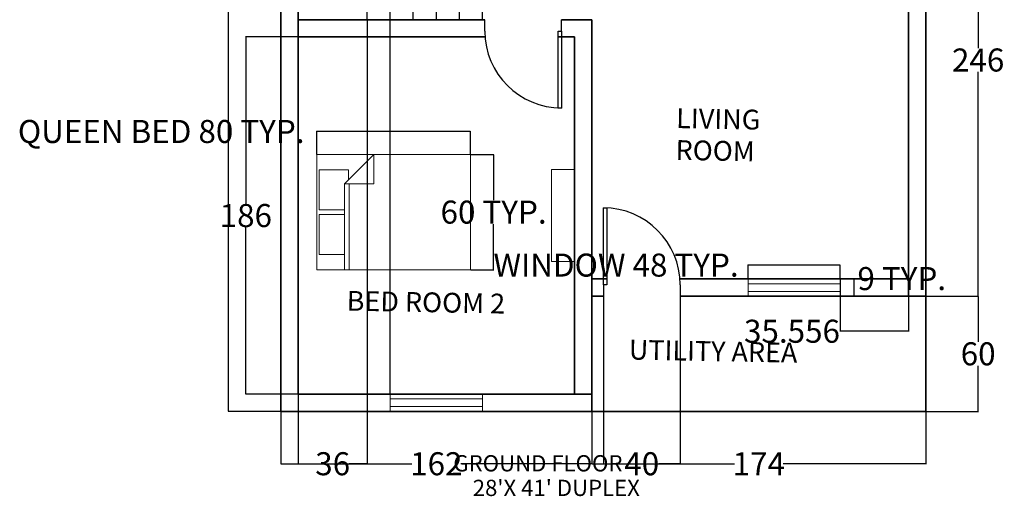
# Model space of a CAD drawing. Units: inches. Extents: x 424 to 1593, y 6 to 578.
# Tile 1 of 4: x 424 to 937, y 6 to 255. Entities that reach past the tile are written whole.
import ezdxf

# ---------------------------------------------------------------- set-up
doc = ezdxf.new("R2010")
doc.units = ezdxf.units.IN
doc.header["$MEASUREMENT"] = 0
for name, color, linetype, lineweight in [('A-ANNO-DIMS', 2, 'Continuous', 18), ('A-ANNO-TEXT', 7, 'Continuous', 25), ('A-AREA-IDEN', 7, 'Continuous', 18), ('A-DOOR', 3, 'Continuous', 25), ('A-FLOR-CASE', 9, 'Continuous', 18), ('A-FLOR-STRS', 7, 'Continuous', 25), ('A-FURN', 8, 'Continuous', 18), ('A-GLAZ', 4, 'Continuous', 18), ('A-WALL', 7, 'Continuous', 35)]:
    doc.layers.add(name, color=color, linetype=linetype, lineweight=lineweight)
doc.styles.get("Standard").update_dxf_attribs({"font": 'arial.ttf'})
doc.dimstyles.get("Standard").update_dxf_attribs({"dimtxt": 12, "dimasz": 0.18, "dimexe": 0.18, "dimexo": 0.0625, "dimgap": 0.09, "dimtad": 0, "dimtih": 1, "dimtoh": 1, "dimdec": 0, "dimzin": 0, "dimdsep": 46, "dimlunit": 3, "dimtxsty": 'Standard', "dimcen": 0.09, "dimadec": 0, "dimazin": 0, "dimtfac": 1, "dimtdec": 0, "dimtofl": 0, "dimtmove": 0, "dimatfit": 3, "dimfxl": 1, "dimtolj": 1, "dimtzin": 0, "dimarcsym": 0})

# ---------------------------------------------------------------- blocks, each defined once
blk = doc.blocks.new('*U4')
for p, q in [((-40, 0), (-40, 6)), ((0, 0), (0, 6))]:
    blk.add_line(p, q)
blk.add_lwpolyline([(0, 0), (0, -40), (-1.75, -40), (-1.75, 0)], close=True)
blk.add_arc((0, 0), 40, 180, 270)
blk = doc.blocks.new('*U6')
for p, q in [((0, 0), (0, -6)), ((40, 0), (40, -6))]:
    blk.add_line(p, q)
blk.add_lwpolyline([(0, 0), (0, 40), (1.75, 40), (1.75, 0)], close=True)
blk.add_arc((0, 0), 40, 0, 90)
blk = doc.blocks.new('Bed - Queen')
for p, q in [((0, -80.00003), (0, 0)), ((0, 0), (59.99999, 0)), ((59.99999, 0), (59.99999, -80.00003)), ((7.99999, -1.2), (28.79998, -1.2)), ((7.99999, -14.4), (7.99999, -1.2)), ((28.79998, -1.2), (28.79998, -14.4)), ((31.19999, -1.2), (51.99999, -1.2)), ((31.19999, -14.4), (31.19999, -1.2)), ((51.99999, -1.2), (51.99999, -16.4)), ((0, -14.4), (44.8, -14.4)), ((59.99999, -29.6), (44.8, -14.4)), ((44.8, -14.4), (44.8, -29.6)), ((44.8, -16.8), (0, -16.8)), ((51.99999, -16.4), (46.79936, -16.4)), ((44.8, -29.6), (59.99999, -29.6)), ((59.99999, -80.00003), (0, -80.00003))]:
    blk.add_line(p, q)
blk = doc.blocks.new('WIN-48IN')
for p, q in [((2.5, 48), (2.5, 0)), ((6.5, 48), (6.5, 0))]:
    blk.add_line(p, q)
blk.add_lwpolyline([(0, 48), (9, 48), (9, 0), (0, 0)], close=True)
blk = doc.blocks.new('STAIR-RETURN-102IN')
for p, q in [((2, 60.44), (2, 102)), ((14, 60.44), (14, 102)), ((26, 60.44), (26, 102)), ((38, 60.44), (38, 102)), ((50, 60.44), (50, 102)), ((62, 60.44), (62, 102)), ((2, 43.56), (2, 58.44)), ((62, 43.56), (62, 58.44)), ((2, 0), (2, 41.56)), ((14, 0), (14, 41.56)), ((26, 0), (26, 41.56)), ((38, 0), (38, 41.56)), ((50, 0), (50, 41.56)), ((62, 0), (62, 41.56))]:
    blk.add_line(p, q)
for points in [[(0, 60.44), (64, 60.44), (64, 41.56), (0, 41.56)], [(2, 58.44), (62, 58.44), (62, 43.56), (2, 43.56)]]:
    blk.add_lwpolyline(points, close=True)
blk = doc.blocks.new('CASEWORK-48X12')
blk.add_lwpolyline([(12, 48), (0, 48), (0, 0), (12, 0)], close=True)
blk = doc.blocks.new('*D12')
at = {"layer": 'A-ANNO-DIMS', "color": 0, "lineweight": -2, "transparency": 16777216}
for p, q in [((803.16, 126.73), (802.98, 126.73)), ((803.16, 119.59), (803.16, 126.91)), ((850.98, 126.73), (803.34, 126.73)), ((851.16, 119.59), (851.16, 126.91))]:
    blk.add_line(p, q, dxfattribs=at)
at = {"layer": 'A-ANNO-DIMS', "color": 0, "transparency": 16777216}
for points in [[(803.34, 126.76), (803.34, 126.7), (803.16, 126.73)], [(850.98, 126.76), (850.98, 126.7), (851.16, 126.73)]]:
    blk.add_solid(points, dxfattribs=at)
at = {"layer": 'Defpoints', "color": 0, "transparency": 16777216}
for p in [(803.16, 126.73), (803.16, 119.53), (851.16, 119.53)]:
    blk.add_point(p, dxfattribs=at)
at = {"layer": 'A-ANNO-DIMS', "color": 0, "transparency": 16777216, "insert": (734.33, 126.73), "char_height": 12, "attachment_point": 5}
blk.add_mtext('\\A1;WINDOW 48 TYP.', dxfattribs=at)
blk = doc.blocks.new('*D13')
at = {"layer": 'A-ANNO-DIMS', "color": 0, "lineweight": -2, "transparency": 16777216}
for p, q in [((851.22, 119.53), (858.54, 119.53)), ((858.36, 119.53), (858.36, 119.71)), ((858.36, 119.71), (858.54, 119.71)), ((858.36, 110.71), (858.36, 119.35)), ((851.22, 110.53), (858.54, 110.53))]:
    blk.add_line(p, q, dxfattribs=at)
at = {"layer": 'A-ANNO-DIMS', "color": 0, "transparency": 16777216}
for points in [[(858.33, 119.35), (858.39, 119.35), (858.36, 119.53)], [(858.33, 110.71), (858.39, 110.71), (858.36, 110.53)]]:
    blk.add_solid(points, dxfattribs=at)
at = {"layer": 'Defpoints', "color": 0, "transparency": 16777216}
for p in [(851.16, 119.53), (858.36, 119.53), (851.16, 110.53)]:
    blk.add_point(p, dxfattribs=at)
at = {"layer": 'A-ANNO-DIMS', "color": 0, "transparency": 16777216, "insert": (883.17, 119.71), "char_height": 12, "attachment_point": 5}
blk.add_mtext('\\A1;9 TYP.', dxfattribs=at)
blk = doc.blocks.new('*D16')
at = {"layer": 'A-ANNO-DIMS', "color": 0, "lineweight": -2, "transparency": 16777216}
for p, q in [((578.54, 196.32), (578.36, 196.32)), ((578.54, 184.38), (578.54, 196.5)), ((658.36, 196.32), (578.72, 196.32)), ((658.54, 184.38), (658.54, 196.5))]:
    blk.add_line(p, q, dxfattribs=at)
at = {"layer": 'A-ANNO-DIMS', "color": 0, "transparency": 16777216}
for points in [[(578.72, 196.35), (578.72, 196.29), (578.54, 196.32)], [(658.36, 196.35), (658.36, 196.29), (658.54, 196.32)]]:
    blk.add_solid(points, dxfattribs=at)
at = {"layer": 'Defpoints', "color": 0, "transparency": 16777216}
for p in [(578.54, 196.32), (578.54, 184.32), (658.54, 184.32)]:
    blk.add_point(p, dxfattribs=at)
at = {"layer": 'A-ANNO-DIMS', "color": 0, "transparency": 16777216, "insert": (497.38, 196.32), "char_height": 12, "attachment_point": 5}
blk.add_mtext('\\A1;QUEEN BED 80 TYP.', dxfattribs=at)
blk = doc.blocks.new('*D17')
at = {"layer": 'A-ANNO-DIMS', "color": 0, "lineweight": -2, "transparency": 16777216}
for p, q in [((658.6, 184.32), (670.72, 184.32)), ((670.54, 184.14), (670.54, 160.54)), ((670.54, 124.5), (670.54, 148.1)), ((658.6, 124.32), (670.72, 124.32))]:
    blk.add_line(p, q, dxfattribs=at)
at = {"layer": 'A-ANNO-DIMS', "color": 0, "transparency": 16777216}
for points in [[(670.51, 184.14), (670.57, 184.14), (670.54, 184.32)], [(670.51, 124.5), (670.57, 124.5), (670.54, 124.32)]]:
    blk.add_solid(points, dxfattribs=at)
at = {"layer": 'Defpoints', "color": 0, "transparency": 16777216}
for p in [(658.54, 184.32), (670.54, 184.32), (658.54, 124.32)]:
    blk.add_point(p, dxfattribs=at)
at = {"layer": 'A-ANNO-DIMS', "color": 0, "transparency": 16777216, "insert": (670.54, 154.32), "char_height": 12, "attachment_point": 5}
blk.add_mtext('\\A1;60 TYP.', dxfattribs=at)
blk = doc.blocks.new('*D23')
at = {"layer": 'A-ANNO-DIMS', "color": 0, "lineweight": -2, "transparency": 16777216}
for p, q in [((559.65, 542.53), (532.29, 542.53)), ((532.47, 542.35), (532.47, 302.75)), ((532.47, 50.71), (532.47, 290.31)), ((559.65, 50.53), (532.29, 50.53))]:
    blk.add_line(p, q, dxfattribs=at)
at = {"layer": 'A-ANNO-DIMS', "color": 0, "transparency": 16777216}
for points in [[(532.44, 542.35), (532.5, 542.35), (532.47, 542.53)], [(532.44, 50.71), (532.5, 50.71), (532.47, 50.53)]]:
    blk.add_solid(points, dxfattribs=at)
at = {"layer": 'Defpoints', "color": 0, "transparency": 16777216}
for p in [(532.47, 542.53), (559.72, 542.53), (559.72, 50.53)]:
    blk.add_point(p, dxfattribs=at)
at = {"layer": 'A-ANNO-DIMS', "color": 0, "transparency": 16777216, "insert": (532.47, 296.53), "char_height": 12, "attachment_point": 5}
blk.add_mtext('\\A1;492', dxfattribs=at)
blk = doc.blocks.new('*D24')
at = {"layer": 'A-ANNO-DIMS', "color": 0, "lineweight": -2, "transparency": 16777216}
for p, q in [((559.72, 50.47), (559.72, 23.1)), ((721.72, 50.47), (721.72, 23.1)), ((559.9, 23.28), (628, 23.28)), ((721.54, 23.28), (653.44, 23.28))]:
    blk.add_line(p, q, dxfattribs=at)
at = {"layer": 'A-ANNO-DIMS', "color": 0, "transparency": 16777216}
for points in [[(559.9, 23.31), (559.9, 23.25), (559.72, 23.28)], [(721.54, 23.31), (721.54, 23.25), (721.72, 23.28)]]:
    blk.add_solid(points, dxfattribs=at)
at = {"layer": 'Defpoints', "color": 0, "transparency": 16777216}
for p in [(559.72, 50.53), (721.72, 50.53), (721.72, 23.28)]:
    blk.add_point(p, dxfattribs=at)
at = {"layer": 'A-ANNO-DIMS', "color": 0, "transparency": 16777216, "insert": (640.72, 23.28), "char_height": 12, "attachment_point": 5}
blk.add_mtext('\\A1;162', dxfattribs=at)
blk = doc.blocks.new('*D25')
at = {"layer": 'A-ANNO-DIMS', "color": 0, "lineweight": -2, "transparency": 16777216}
for p, q in [((721.72, 50.47), (721.72, 23.1)), ((895.72, 50.47), (895.72, 23.1)), ((721.9, 23.28), (795.96, 23.28)), ((895.54, 23.28), (821.47, 23.28))]:
    blk.add_line(p, q, dxfattribs=at)
at = {"layer": 'A-ANNO-DIMS', "color": 0, "transparency": 16777216}
for points in [[(721.9, 23.31), (721.9, 23.25), (721.72, 23.28)], [(895.54, 23.31), (895.54, 23.25), (895.72, 23.28)]]:
    blk.add_solid(points, dxfattribs=at)
at = {"layer": 'Defpoints', "color": 0, "transparency": 16777216}
for p in [(721.72, 50.53), (895.72, 50.53), (895.72, 23.28)]:
    blk.add_point(p, dxfattribs=at)
at = {"layer": 'A-ANNO-DIMS', "color": 0, "transparency": 16777216, "insert": (808.72, 23.28), "char_height": 12, "attachment_point": 5}
blk.add_mtext('\\A1;174', dxfattribs=at)
blk = doc.blocks.new('*D26')
at = {"layer": 'A-ANNO-DIMS', "color": 0, "lineweight": -2, "transparency": 16777216}
for p, q in [((568.65, 245.53), (541.29, 245.53)), ((541.47, 245.35), (541.47, 158.75)), ((541.47, 59.71), (541.47, 146.31)), ((568.65, 59.53), (541.29, 59.53))]:
    blk.add_line(p, q, dxfattribs=at)
at = {"layer": 'A-ANNO-DIMS', "color": 0, "transparency": 16777216}
for points in [[(541.44, 245.35), (541.5, 245.35), (541.47, 245.53)], [(541.44, 59.71), (541.5, 59.71), (541.47, 59.53)]]:
    blk.add_solid(points, dxfattribs=at)
at = {"layer": 'Defpoints', "color": 0, "transparency": 16777216}
for p in [(541.47, 245.53), (568.72, 245.53), (568.72, 59.53)]:
    blk.add_point(p, dxfattribs=at)
at = {"layer": 'A-ANNO-DIMS', "color": 0, "transparency": 16777216, "insert": (541.47, 152.53), "char_height": 12, "attachment_point": 5}
blk.add_mtext('\\A1;186', dxfattribs=at)
blk = doc.blocks.new('*D28')
at = {"layer": 'A-ANNO-DIMS', "color": 0, "lineweight": -2, "transparency": 16777216}
for p, q in [((895.78, 110.53), (923.15, 110.53)), ((922.97, 110.35), (922.97, 86.75)), ((922.97, 50.71), (922.97, 74.31)), ((895.78, 50.53), (923.15, 50.53))]:
    blk.add_line(p, q, dxfattribs=at)
at = {"layer": 'A-ANNO-DIMS', "color": 0, "transparency": 16777216}
for points in [[(922.94, 110.35), (923, 110.35), (922.97, 110.53)], [(922.94, 50.71), (923, 50.71), (922.97, 50.53)]]:
    blk.add_solid(points, dxfattribs=at)
at = {"layer": 'Defpoints', "color": 0, "transparency": 16777216}
for p in [(895.72, 110.53), (922.97, 110.53), (895.72, 50.53)]:
    blk.add_point(p, dxfattribs=at)
at = {"layer": 'A-ANNO-DIMS', "color": 0, "transparency": 16777216, "insert": (922.97, 80.53), "char_height": 12, "attachment_point": 5}
blk.add_mtext('\\A1;60', dxfattribs=at)
blk = doc.blocks.new('*D29')
at = {"layer": 'A-ANNO-DIMS', "color": 0, "lineweight": -2, "transparency": 16777216}
for p, q in [((886.78, 356.53), (923.15, 356.53)), ((922.97, 356.35), (922.97, 239.75)), ((922.97, 110.71), (922.97, 227.31)), ((895.78, 110.53), (923.15, 110.53))]:
    blk.add_line(p, q, dxfattribs=at)
at = {"layer": 'A-ANNO-DIMS', "color": 0, "transparency": 16777216}
for points in [[(922.94, 356.35), (923, 356.35), (922.97, 356.53)], [(922.94, 110.71), (923, 110.71), (922.97, 110.53)]]:
    blk.add_solid(points, dxfattribs=at)
at = {"layer": 'Defpoints', "color": 0, "transparency": 16777216}
for p in [(886.72, 356.53), (922.97, 356.53), (895.72, 110.53)]:
    blk.add_point(p, dxfattribs=at)
at = {"layer": 'A-ANNO-DIMS', "color": 0, "transparency": 16777216, "insert": (922.97, 233.53), "char_height": 12, "attachment_point": 5}
blk.add_mtext('\\A1;246', dxfattribs=at)
blk = doc.blocks.new('*D32')
at = {"layer": 'A-ANNO-DIMS', "color": 0, "lineweight": -2, "transparency": 16777216}
for p, q in [((568.72, 59.59), (568.72, 569.96)), ((568.9, 569.78), (583.78, 569.78)), ((616.54, 569.78), (601.65, 569.78)), ((616.72, 59.59), (616.72, 569.96))]:
    blk.add_line(p, q, dxfattribs=at)
at = {"layer": 'A-ANNO-DIMS', "color": 0, "transparency": 16777216}
for points in [[(568.9, 569.81), (568.9, 569.75), (568.72, 569.78)], [(616.54, 569.81), (616.54, 569.75), (616.72, 569.78)]]:
    blk.add_solid(points, dxfattribs=at)
at = {"layer": 'Defpoints', "color": 0, "transparency": 16777216}
for p in [(616.72, 569.78), (568.72, 59.53), (616.72, 59.53)]:
    blk.add_point(p, dxfattribs=at)
at = {"layer": 'A-ANNO-DIMS', "color": 0, "transparency": 16777216, "insert": (592.72, 569.78), "char_height": 12, "attachment_point": 5}
blk.add_mtext('\\A1;48', dxfattribs=at)
blk = doc.blocks.new('*D33')
at = {"layer": 'A-ANNO-DIMS', "color": 0, "lineweight": -2, "transparency": 16777216}
for p, q in [((727.72, 110.47), (727.72, 23.1)), ((767.72, 110.47), (767.72, 23.1)), ((727.9, 23.28), (738.81, 23.28)), ((767.54, 23.28), (756.62, 23.28))]:
    blk.add_line(p, q, dxfattribs=at)
at = {"layer": 'A-ANNO-DIMS', "color": 0, "transparency": 16777216}
for points in [[(727.9, 23.31), (727.9, 23.25), (727.72, 23.28)], [(767.54, 23.31), (767.54, 23.25), (767.72, 23.28)]]:
    blk.add_solid(points, dxfattribs=at)
at = {"layer": 'Defpoints', "color": 0, "transparency": 16777216}
for p in [(727.72, 110.53), (767.72, 110.53), (767.72, 23.28)]:
    blk.add_point(p, dxfattribs=at)
at = {"layer": 'A-ANNO-DIMS', "color": 0, "transparency": 16777216, "insert": (747.72, 23.28), "char_height": 12, "attachment_point": 5}
blk.add_mtext('\\A1;40', dxfattribs=at)
blk = doc.blocks.new('*D34')
at = {"layer": 'A-ANNO-DIMS', "color": 0, "lineweight": -2, "transparency": 16777216}
for p, q in [((568.72, 254.47), (568.72, 23.1)), ((604.72, 254.47), (604.72, 23.1)), ((568.9, 23.28), (578.04, 23.28)), ((604.54, 23.28), (595.39, 23.28))]:
    blk.add_line(p, q, dxfattribs=at)
at = {"layer": 'A-ANNO-DIMS', "color": 0, "transparency": 16777216}
for points in [[(568.9, 23.31), (568.9, 23.25), (568.72, 23.28)], [(604.54, 23.31), (604.54, 23.25), (604.72, 23.28)]]:
    blk.add_solid(points, dxfattribs=at)
at = {"layer": 'Defpoints', "color": 0, "transparency": 16777216}
for p in [(568.72, 254.53), (604.72, 254.53), (604.72, 23.28)]:
    blk.add_point(p, dxfattribs=at)
at = {"layer": 'A-ANNO-DIMS', "color": 0, "transparency": 16777216, "insert": (586.72, 23.28), "char_height": 12, "attachment_point": 5}
blk.add_mtext('\\A1;36', dxfattribs=at)
blk = doc.blocks.new('*D40')
at = {"layer": 'A-ANNO-DIMS', "color": 0, "lineweight": -2, "transparency": 16777216}
for p, q in [((851.16, 119.47), (851.16, 92.1)), ((886.72, 119.47), (886.72, 92.1)), ((851.16, 92.28), (850.98, 92.28)), ((886.54, 92.28), (851.34, 92.28))]:
    blk.add_line(p, q, dxfattribs=at)
at = {"layer": 'A-ANNO-DIMS', "color": 0, "transparency": 16777216}
for points in [[(851.34, 92.31), (851.34, 92.25), (851.16, 92.28)], [(886.54, 92.31), (886.54, 92.25), (886.72, 92.28)]]:
    blk.add_solid(points, dxfattribs=at)
at = {"layer": 'Defpoints', "color": 0, "transparency": 16777216}
for p in [(851.16, 119.53), (886.72, 119.53), (851.16, 92.28)]:
    blk.add_point(p, dxfattribs=at)
at = {"layer": 'A-ANNO-DIMS', "color": 0, "transparency": 16777216, "insert": (825.99, 92.28), "char_height": 12, "attachment_point": 5}
blk.add_mtext('\\A1;35.556', dxfattribs=at)

msp = doc.modelspace()

# ---------------------------------------------------------------- linework, layer by layer
at = {"layer": 'A-WALL'}
for p, q in [((886.7159, 533.5296), (886.7159, 110.5296)), ((568.7159, 254.5296), (568.7159, 356.5296)), ((568.7159, 254.5296), (665.9977, 254.5296)), ((705.9977, 254.5296), (711.9977, 254.5296)), ((705.9977, 254.5296), (721.7159, 254.5296)), ((721.7159, 50.5296), (721.7159, 254.5296)), ((568.7159, 59.5296), (568.7159, 245.5296)), ((568.7159, 245.5296), (666.1104, 245.5296)), ((704.2477, 245.5296), (712.7159, 245.5296)), ((712.7159, 59.5296), (712.7159, 245.5296)), ((721.7159, 119.5296), (729.4659, 119.5296)), ((767.6033, 119.5296), (886.7159, 119.5296)), ((721.7159, 110.5296), (727.7159, 110.5296)), ((727.7159, 110.5296), (721.7159, 110.5296)), ((767.7159, 110.5296), (895.7159, 110.5296)), ((895.7159, 110.5296), (895.7159, 50.5296)), ((721.7159, 59.5296), (568.7159, 59.5296)), ((721.7159, 50.5296), (895.7159, 50.5296))]:
    msp.add_line(p, q, dxfattribs=at)
msp.add_lwpolyline([(721.7159, 50.5296), (559.7159, 50.5296), (559.7159, 542.5296), (895.7159, 542.5296), (895.7159, 110.5296)], dxfattribs=at)

# ---------------------------------------------------------------- block references
at = {"layer": 'A-DOOR'}
for name, p in [('*U4', (705.9977, 248.5296)), ('*U6', (727.7159, 116.5296))]:
    msp.add_blockref(name, p, dxfattribs=at)
at = {"layer": 'A-FLOR-CASE'}
msp.add_blockref('CASEWORK-48X12', (700.716, 128.5295), dxfattribs=at)
at = {"layer": 'A-FLOR-STRS'}
msp.add_blockref('STAIR-RETURN-102IN', (602.716, 254.53), dxfattribs=at)
at = {"layer": 'A-FURN', "rotation": 90}
msp.add_blockref('Bed - Queen', (578.5402, 124.3181), dxfattribs=at)
at = {"layer": 'A-GLAZ'}
for p, rotation in [((851.1597, 110.5297), 90), ((664.716, 50.5297), 89.99999999999996)]:
    msp.add_blockref('WIN-48IN', p, dxfattribs=dict(at, rotation=rotation))

# ---------------------------------------------------------------- texts
at = {"layer": 'A-ANNO-TEXT'}
for s, p in [('GROUND FLOOR', (649.5901, 19.2803)), ("28'X 41' DUPLEX", (659.6989, 6.4728))]:
    msp.add_text(s, height=8.45662, dxfattribs=at).set_placement(p)
at = {"layer": 'A-AREA-IDEN'}
for s, height, p in [('LIVING', 10.30671, (765.5853, 198.1025)), ('ROOM', 10.30671, (765.272, 181.5486)), ('BED ROOM 2', 10.30671, (593.9427, 103.024)), ('UTILITY AREA', 10.306713, (740.9435, 77.5565))]:
    msp.add_text(s, height=height, rotation=358.915866, dxfattribs=at).set_placement(p)

# ---------------------------------------------------------------- dimensions: what is measured, and where the dimension line sits
at = {"layer": 'A-ANNO-DIMS'}
for base, p1, p2, picture, middle in [((616.7159, 569.7796), (568.7159, 59.5296), (616.7159, 59.5296), '*D32', (592.7159, 569.7796)), ((604.7159, 23.2796), (568.7159, 254.5296), (604.7159, 254.5296), '*D34', (586.7159, 23.2796)), ((767.7159, 23.2796), (727.7159, 110.5296), (767.7159, 110.5296), '*D33', (747.7159, 23.2796)), ((721.7159, 23.2796), (559.7159, 50.5296), (721.7159, 50.5296), '*D24', (640.7159, 23.2796)), ((895.7159, 23.2796), (721.7159, 50.5296), (895.7159, 50.5296), '*D25', (808.7159, 23.2796))]:
    dim = msp.add_linear_dim(base=base, p1=p1, p2=p2, dimstyle='Standard', override={"dimdec": 0, "dimlfac": 1, "dimrnd": 0, "dimzin": 0, "dimdsep": 46, "dimlunit": 2}, dxfattribs=at)
    dim.commit()
    dim.dimension.update_dxf_attribs({"geometry": picture, "text_midpoint": middle})
for base, p1, p2, angle, override, picture, middle in [((532.4659, 542.5296), (559.7159, 50.5296), (559.7159, 542.5296), 90, {"dimdec": 0, "dimlfac": 1, "dimrnd": 0, "dimzin": 0, "dimdsep": 46, "dimlunit": 2}, '*D23', (532.4659, 296.5296)), ((922.9659, 356.5296), (895.7159, 110.5296), (886.7159, 356.5296), 90, {"dimdec": 0, "dimlfac": 1, "dimrnd": 0, "dimzin": 0, "dimdsep": 46, "dimlunit": 2}, '*D29', (922.9659, 233.5296)), ((541.4659, 245.5296), (568.7159, 59.5296), (568.7159, 245.5296), 90, {"dimdec": 0, "dimlfac": 1, "dimrnd": 0, "dimzin": 0, "dimdsep": 46, "dimlunit": 2}, '*D26', (541.4659, 152.5296)), ((851.1596, 92.2796), (886.7159, 119.5296), (851.1596, 119.5296), 180, {"dimdec": 3, "dimlfac": 1, "dimrnd": 0, "dimzin": 0, "dimdsep": 46, "dimlunit": 2}, '*D40', (825.9892, 92.2796)), ((922.9659, 110.5296), (895.7159, 50.5296), (895.7159, 110.5296), 90, {"dimdec": 0, "dimlfac": 1, "dimrnd": 0, "dimzin": 0, "dimdsep": 46, "dimlunit": 2}, '*D28', (922.9659, 80.5296))]:
    dim = msp.add_linear_dim(base=base, p1=p1, p2=p2, angle=angle, dimstyle='Standard', override=override, dxfattribs=at)
    dim.commit()
    dim.dimension.update_dxf_attribs({"geometry": picture, "text_midpoint": middle})
for base, p1, p2, angle, text, picture, middle in [((578.5402, 196.3181), (658.5402, 184.3181), (578.5402, 184.3181), 180, 'QUEEN BED <> TYP.', '*D16', (497.3766, 196.3181)), ((670.5402, 184.3181), (658.5402, 124.3181), (658.5402, 184.3181), 90, '<> TYP.', '*D17', (670.5402, 154.3181)), ((803.1596, 126.7296), (851.1596, 119.5296), (803.1596, 119.5296), 180, 'WINDOW <> TYP.', '*D12', (734.3316, 126.7296)), ((858.3596, 119.5296), (851.1596, 110.5296), (851.1596, 119.5296), 90, '<> TYP.', '*D13', (883.1739, 119.7096))]:
    dim = msp.add_linear_dim(base=base, p1=p1, p2=p2, angle=angle, text=text, dimstyle='Standard', override={"dimdec": 0, "dimlfac": 1, "dimrnd": 0, "dimzin": 0, "dimdsep": 46, "dimlunit": 2}, dxfattribs=at)
    dim.commit()
    dim.dimension.update_dxf_attribs({"geometry": picture, "text_midpoint": middle})

doc.saveas('drawing.dxf')
